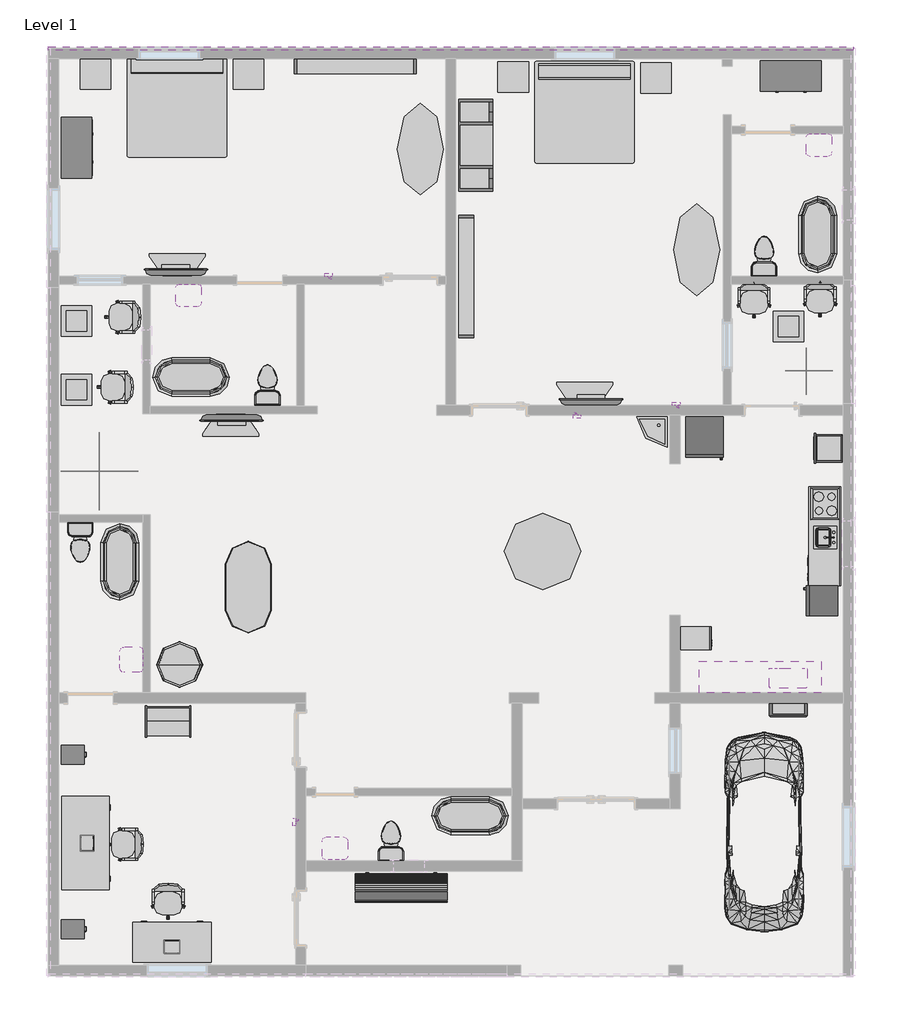
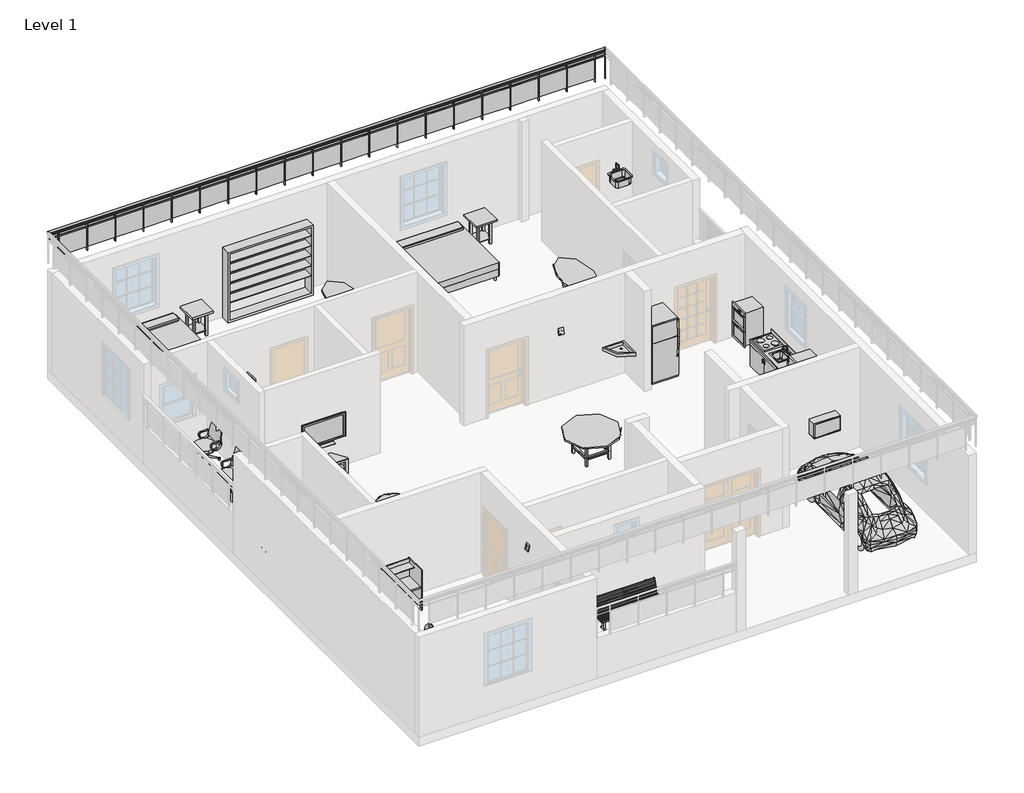
# One storey, part 4 of 4: 37 furniture elements, 17 proxies, 14 flow terminals, 3 geographic elements, 1 railing.
# Revit data of these elements (continued)
# Type "Shelving : 96\" x 12\" x 84\"" (continued)
#   Shelving Unit Material = Laminate, Ivory, Matte
#   Default Elevation = 0
# Type "TV - Flat Screen : 50\""
#   SinAng = 0' - 0.0193"
#   L = 3' - 7.57782"
#   H = 2' - 0.51477"
#   Thickness = 0' - 4.33071"
#   Diagonal = 4' - 2"
#   CosAng = 0' - 0.03431"
#   Stand [instance default] = yes
#   Default Elevation = 0
# Type "TV Stand : TV Stand"
#   Depth = 1' - 6"
#   Width = 3' - 8"
#   Height = 1' - 7 1/2"
#   Finish = Melamine - Gray
#   Default Elevation = 0
# Type "Table-Coffee : 24\" x 24\" x 24\""
#   Assembly Code = "E2020200"
#   Height = 2' - 0"
#   Length = 2' - 0"
#   Width = 2' - 0"
#   Top Material = none
#   Frame Material = none
#   Default Elevation = 0
# Type "Table-Dining Oval : 36\" x 72\""
#   Assembly Code = "E2020200"
#   Length = 6' - 0"
#   Width = 3' - 0"
#   Base Material = Steel, Chrome Plated
#   Top Material = Glass - Clear, Grey
#   Default Elevation = 0
#   Description = (empty or 0)
# Type "Table-Dining Round w Chairs : 60\" Diameter"
#   Assembly Code = "E2020200"
#   Radius = 2' - 6"
#   Diameter = 5' - 0"
#   Height = 2' - 6"
#   Chairs = 6
#   Base Material = Pine
#   Top Material = Laminate, Linen, Matte
#   Default Elevation = 0
# Type "Table-Ellipse : 72\" x 36\""
#   Assembly Code = "E2020200"
#   Half Width = 1' - 6"
#   Half Length = 3' - 0"
#   Height = 2' - 6"
#   Length = 6' - 0"
#   Width = 3' - 0"
#   Base Material = Birch
#   Top Material = Laminate - Black
#   Default Elevation = 0
# Type "Table-Night Stand : 24\" x 24\" x 30\""
#   Assembly Code = "E2020200"
#   Depth = 2' - 0"
#   Height = 2' - 6"
#   Width = 2' - 0"
#   Base Material = Birch
#   Top Material = Laminate, Ivory, Matte
#   Default Elevation = 0
# Type "Table-Round : 36\" Diameter"
#   Assembly Code = "E2020200"
#   Base Radius = 0' - 10"
#   Height = 2' - 6"
#   Radius = 1' - 6"
#   Base Material = Steel, Chrome Plated
#   Top Material = Birch
#   Default Elevation = 0
# Type "Park Bench : 72\""
#   Length = 6' - 0"
#   Seat Material = Wood - Teak
#   Frame Material = Steel, Paint Finish, Dark Gray, Matte
# Type "RPC Shrub : Burning Bush 4'-6\""
#   Type Comments = "Burning Bush"
#   built-in parameter 1005198 = "{2, 15},{39, RPC-16-FVGW-0UXX-7JA7-N000-ST1L-LVER-AU},{1, 0},{1, 0},{2, 13},{1, 8},{5, Color},{1, 0},{1, 0},{3, 0.8},{3, 0.8},{3, 0.8},{1, 8},{7, BBoxMin},{1, 0},{1, 0},{1, 0},{1, 0},{1, 0},{1, 8},{7, BBoxMax},{1, 0},{1, 0},{1, 0},{1, 0},{1, 0},{2, 11},{9, RPCTypeId},{1, 0},{1, 0},{39, RPC-16-FVGW-0UXX-7JA7-N000-ST1L-LVER-AU},{1, 6},{14, RPCPlantHeight},{1, 0},{1, 0},{3, 4.5},{2, 11},{7, keyword},{1, 0},{1, 0},{35, :RPCs:Shrubs & Grasses:Geometry:RPC},{2, 11},{8, category},{1, 0},{1, 0},{16, Shrubs & Grasses},{2, 11},{12, LocalizedUID},{1, 0},{1, 0},{12, Burning Bush},{2, 14},{6, Height},{1, 0},{1, 0},{3, 4.5},{1, 2},{16, Cast Reflections},{1, 0},{1, 0},{1, 0},{1, 2},{12, Cast Shadows},{1, 0},{1, 0},{1, 1},{1, 2},{9, Lock View},{1, 0},{1, 0},{1, 0},{1, 4},{5, ViewC},{1, 0},{1, 0},{1, 0},{21, assetlibrary_base.fbx},{1, 5},"
#   built-in parameter 1005195 = "RPC-16-FVGW-0UXX-7JA7-N000-ST1L-LVER-AU"
#   Assembly Code = "G2050500"
#   Height = 4' - 6"
#   Default Elevation = 0
# Type "RPC Shrub : Cedar Shrub 3'-0\""
#   Type Comments = "Cedar Shrub"
#   built-in parameter 1005198 = "{2, 15},{39, RPC-16-FUMD-ULXX-U7X6-J000-ST1L-LVER-AU},{1, 0},{1, 0},{2, 13},{1, 8},{5, Color},{1, 0},{1, 0},{3, 0.8},{3, 0.8},{3, 0.8},{1, 8},{7, BBoxMin},{1, 0},{1, 0},{1, 0},{1, 0},{1, 0},{1, 8},{7, BBoxMax},{1, 0},{1, 0},{1, 0},{1, 0},{1, 0},{2, 11},{9, RPCTypeId},{1, 0},{1, 0},{39, RPC-16-FUMD-ULXX-U7X6-J000-ST1L-LVER-AU},{1, 6},{14, RPCPlantHeight},{1, 0},{1, 0},{1, 3},{2, 11},{7, keyword},{1, 0},{1, 0},{35, :RPCs:Shrubs [General]:Geometry:RPC},{2, 11},{8, category},{1, 0},{1, 0},{16, Shrubs [General]},{2, 11},{12, LocalizedUID},{1, 0},{1, 0},{11, Cedar Shrub},{2, 14},{6, Height},{1, 0},{1, 0},{1, 3},{1, 2},{16, Cast Reflections},{1, 0},{1, 0},{1, 0},{1, 2},{12, Cast Shadows},{1, 0},{1, 0},{1, 1},{1, 2},{9, Lock View},{1, 0},{1, 0},{1, 0},{1, 4},{5, ViewC},{1, 0},{1, 0},{1, 0},{21, assetlibrary_base.fbx},{1, 5},"
#   built-in parameter 1005195 = "RPC-16-FUMD-ULXX-U7X6-J000-ST1L-LVER-AU"
#   Assembly Code = "G2050500"
#   Height = 3' - 0"
#   Default Elevation = 0
# Type "Glass Panel - Bottom Fill"
#   Assembly Code = "C2010400"
#   built-in parameter 1008612 = 0.0416667 (stored number, unit not read)
#   built-in parameter 1008611 = 0.0416667 (stored number, unit not read)
#   built-in parameter 1008609 = 0.333333 (stored number, unit not read)
#   built-in parameter 1008604 = 0.166667 (stored number, unit not read)
#   built-in parameter 1008603 = 0.166667 (stored number, unit not read)
#   Railing Height = 3' - 0"
#   built-in parameter 1008630 = 2
#   built-in parameter 1008610 = 2
#   built-in parameter 1008618 = Baluster - Square : 3/4"
# Elements 1, 2 (IfcBuildingElementProxy)
#   Phase Created = New Construction
# Element 3 (IfcBuildingElementProxy, "18\" x 24\" x 34 1/2\"")
#   Phase Created = New Construction
#   Materials on its faces: "Steel, Paint Finish, Ivory, Matte", "Plastic, Opaque Black"
# Element 4 (IfcBuildingElementProxy, "Cook Top-4 Unit2 : 22\" x 20\"")
#   Phase Created = New Construction
#   Materials on its faces: "Steel, Chrome Plated", "Steel, Polished"
# Element 5 (IfcBuildingElementProxy, "Dishwasher : 24\" x 24\" x 34\"")
#   Phase Created = New Construction
#   Materials on its faces: "Steel, Paint Finish, Ivory, Glossy", "Plastic, Opaque Black"
# Element 6 (IfcBuildingElementProxy, "Kitchenette - Medium : Kitchenette - Medium")
#   Phase Created = New Construction
#   Materials on its faces: "Cabinets", "Cabinets - Handles"
# Elements 7, 8 (IfcBuildingElementProxy, "Microwave : 30\" x 16\" x 18\"")
#   Phase Created = New Construction
#   Materials on its faces: "Laminate, Ivory, Matte", "Glass"
# Element 9 (IfcBuildingElementProxy, "Oven Double-Built-in : 21 1/2\" x 39 1/4\" x 21\"")
#   Phase Created = New Construction
#   Materials on its faces: "Steel", "Metal - Stainless Steel, Polished", "Glass"
# Element 10 (IfcBuildingElementProxy, "RPC Beetle : RPC Beetle")
#   Phase Created = New Construction
# Elements 11, 12, 13, 14 (IfcBuildingElementProxy, "RPC Picture Frame : RPC Picture Frame")
#   Phase Created = New Construction
# Element 15 (IfcBuildingElementProxy, "Refrigerator : 24\" x 25\" LH")
#   Phase Created = New Construction
#   Materials on its faces: "Steel, Paint Finish, Ivory, Glossy", "Steel, Chrome Plated"
# Element 16 (IfcBuildingElementProxy, "Refrigerator.0001 : 30\" x 32\" RH")
#   Phase Created = New Construction
#   Materials on its faces: "Steel, Paint Finish, Ivory, Glossy", "Steel, Chrome Plated"
# Element 17 (IfcBuildingElementProxy, "Single Carrel : Single Carrel")
#   Phase Created = New Construction
#   Materials on its faces: "Laminate, Ivory, Matte", "Cherry"
# Element 18 (IfcFlowTerminal, "Sink - Corner Floor : 24\"")
#   Mark = "14"
#   Phase Created = New Construction
# Element 19 (IfcFlowTerminal, "Sink Kitchen-Island : 18\" x 18\"")
#   Mark = "15"
#   Phase Created = New Construction
#   Materials on its faces: "Steel, Polished"
# Element 20 (IfcFlowTerminal, "Sink Vanity-Square : 20\" x 18\"")
#   Mark = "1"
#   Phase Created = New Construction
#   Materials on its faces: "Porcelain, Linen", "Steel, Polished"
# Element 21 (IfcFlowTerminal, "Sink Vanity-Square : 20\" x 18\"")
#   Mark = "2"
#   Phase Created = New Construction
#   Materials on its faces: "Porcelain, Linen", "Steel, Polished"
# Element 22 (IfcFlowTerminal, "Sink Vanity-Square : 20\" x 18\"")
#   Mark = "9"
#   Phase Created = New Construction
#   Materials on its faces: "Porcelain, Linen", "Steel, Polished"
# Element 23 (IfcFlowTerminal, "Sink Vanity-Square : 20\" x 18\"")
#   Mark = "16"
#   Phase Created = New Construction
#   Materials on its faces: "Porcelain, Linen", "Steel, Polished"
# Element 24 (IfcFlowTerminal, "Toilet-Domestic-3D : Toilet-Domestic-3D")
#   Mark = "6"
#   Phase Created = New Construction
#   Materials on its faces: "Porcelain, Linen", "Laminate, Linen, Matte"
# Element 25 (IfcFlowTerminal, "Toilet-Domestic-3D : Toilet-Domestic-3D")
#   Mark = "7"
#   Phase Created = New Construction
#   Materials on its faces: "Porcelain, Linen", "Laminate, Linen, Matte"
# Element 26 (IfcFlowTerminal, "Toilet-Domestic-3D : Toilet-Domestic-3D")
#   Mark = "8"
#   Phase Created = New Construction
#   Materials on its faces: "Porcelain, Linen", "Laminate, Linen, Matte"
# Element 27 (IfcFlowTerminal, "Toilet-Domestic-3D : Toilet-Domestic-3D")
#   Mark = "19"
#   Phase Created = New Construction
#   Materials on its faces: "Porcelain, Linen", "Laminate, Linen, Matte"
# Element 28 (IfcFlowTerminal, "Tub-Free Standing-3D : 30\" x 60\"")
#   Mark = "3"
#   Phase Created = New Construction
#   Materials on its faces: "Porcelain, Ivory"
# Element 29 (IfcFlowTerminal, "Tub-Free Standing-3D : 30\" x 60\"")
#   Mark = "4"
#   Phase Created = New Construction
#   Materials on its faces: "Porcelain, Ivory"
# Element 30 (IfcFlowTerminal, "Tub-Free Standing-3D : 30\" x 60\"")
#   Mark = "11"
#   Phase Created = New Construction
#   Materials on its faces: "Porcelain, Ivory"
# Element 31 (IfcFlowTerminal, "Tub-Free Standing-3D : 30\" x 60\"")
#   Mark = "17"
#   Phase Created = New Construction
#   Materials on its faces: "Porcelain, Ivory"
# Elements 32, 33 (IfcFurniture, "Bed-Standard.0001 : King 78\" x 80\"")
#   Phase Created = New Construction
#   Materials on its faces: "Linen, White", "Steel, Chrome Plated"
# Elements 34, 35 (IfcFurniture, "Cabinet-File 5 Drawer : 15\" x 18\"")
#   Phase Created = New Construction
#   Materials on its faces: "Steel, Chrome Plated", "Steel, Paint Finish, Ivory, Glossy"
# Elements 36, 37, 38, 39, 40, 41 (IfcFurniture, "Chair-Executive : Chair-Executive")
#   Phase Created = New Construction
#   Materials on its faces: "Plastic, Opaque Black", "Textile - Slate Blue"
# Element 42 (IfcFurniture, "Counter Top w Sink Hole : 24\" Depth")
#   Sink Opening Width = 2' - 3"
#   Sink Opening Depth = 1' - 3"
#   Sink Location To Wall = 0' - 6"
#   Sink Location = 2' - 0"
#   Length = 8' - 0"
#   Phase Created = New Construction
#   Materials on its faces: "Counter Top"
# Element 43 (IfcFurniture, "Counter Top w Sink Hole : 24\" Depth")
#   Sink Opening Depth = 1' - 2"
#   Sink Location To Wall = 0' - 6"
#   Length = 6' - 6"
#   Sink Location = 3' - 4"
#   Sink Opening Width = 1' - 4"
#   Phase Created = New Construction
#   Materials on its faces: "Counter Top"
# Element 44 (IfcFurniture, "Desk : 60\" x 30\" Student")
#   Phase Created = New Construction
#   Materials on its faces: "Steel, Chrome Plated", "Laminate, Ivory, Matte", "Cherry"
# Element 45 (IfcFurniture, "Desk : 72\" x 36\"")
#   Phase Created = New Construction
#   Materials on its faces: "Steel, Chrome Plated", "Laminate, Ivory, Matte", "Cherry"
# Elements 46, 47 (IfcFurniture, "Dresser : 48\" x 72\" x 24\"")
#   Phase Created = New Construction
#   Materials on its faces: "Laminate, Ivory, Matte", "Cherry", "Laminate - Ivory, Glossy"
# Element 48 (IfcFurniture, "Entertainment Center : 72\" x 72\" x 24\"")
#   Phase Created = New Construction
#   Materials on its faces: "Steel, Chrome Plated", "Glass - Clear, Grey"
# Elements 49, 50 (IfcFurniture, "Shelving : 96\" x 12\" x 84\"")
#   Phase Created = New Construction
#   Materials on its faces: "Laminate, Ivory, Matte"
# Elements 51, 52, 53 (IfcFurniture, "TV - Flat Screen : 50\"")
#   Stand = yes
#   Phase Created = New Construction
#   Materials on its faces: "TV - Black", "TV - Glass", "TV - Screen"
# Elements 54, 55, 56 (IfcFurniture, "TV Stand : TV Stand")
#   Phase Created = New Construction
#   Materials on its faces: "Melamine - Gray", "Glass - Shelves"
# Elements 57, 58, 59 (IfcFurniture, "Table-Coffee : 24\" x 24\" x 24\"")
#   Phase Created = New Construction
#   Materials on its faces: "Glass - Clear, Grey"
# Element 60 (IfcFurniture, "Table-Dining Oval : 36\" x 72\"")
#   Phase Created = New Construction
#   Materials on its faces: "Steel, Chrome Plated", "Glass - Clear, Grey"
# Element 61 (IfcFurniture, "Table-Dining Round w Chairs : 60\" Diameter")
#   Phase Created = New Construction
#   Materials on its faces: "Pine", "Laminate, Linen, Matte"
# Elements 62, 63 (IfcFurniture, "Table-Ellipse : 72\" x 36\"")
#   Phase Created = New Construction
#   Materials on its faces: "Birch", "Laminate - Black"
# Elements 64, 65, 66, 67 (IfcFurniture, "Table-Night Stand : 24\" x 24\" x 30\"")
#   Phase Created = New Construction
#   Materials on its faces: "Birch", "Laminate, Ivory, Matte"
# Element 68 (IfcFurniture, "Table-Round : 36\" Diameter")
#   Phase Created = New Construction
#   Materials on its faces: "Steel, Chrome Plated", "Birch"
# Element 69 (IfcGeographicElement, "Park Bench : 72\"")
#   Phase Created = New Construction
#   Materials on its faces: "Wood - Teak", "Steel, Paint Finish, Dark Gray, Matte"
# Element 70 (IfcGeographicElement, "RPC Shrub : Burning Bush 4'-6\"")
#   Phase Created = New Construction
# Element 71 (IfcGeographicElement, "RPC Shrub : Cedar Shrub 3'-0\"")
#   Phase Created = New Construction
# Element 72 (IfcRailing, "Glass Panel - Bottom Fill")
#   built-in parameter 1008621 = 10.6667 (stored number, unit not read)
#   Phase Created = New Construction
#   Materials on its faces: "Glass"
# Materials
#   "Plastic, Opaque Black": class "Plastic", colour RGB 0 0 0, transparency 0, Description = "Plastic, generic, opaque black", Cost = 0
#   "Steel, Paint Finish, Ivory, Matte": class "Metal", colour RGB 247 247 239, transparency 0, Description = "Steel, paint finish, ivory, matte", Cost = 0
#   "Steel, Chrome Plated": class "Metal", colour RGB 17 17 17, transparency 0, Description = "Chromiuim plated steel", Cost = 0
#   "Steel, Polished": class "Metal", colour RGB 57 57 57, transparency 0, Description = "Polished steel", Cost = 0
#   "Steel, Paint Finish, Ivory, Glossy": class "Metal", colour RGB 247 247 239, transparency 0, Description = "Steel, paint finish, ivory, glossy", Cost = 0
#   "Cabinets": colour RGB 249 249 249, transparency 0
#   "Cabinets - Handles": class "Metal", colour RGB 57 57 57, transparency 0
#   "Laminate, Ivory, Matte": class "Plastic", colour RGB 247 247 239, transparency 0, Description = "Plastic Laminate - Ivory, Matte", Cost = 0
#   "Metal - Stainless Steel, Polished": class "Metal", colour RGB 216 216 216, transparency 0
#   "Cherry": class "Wood", colour RGB 226 177 128, transparency 0, Description = "Prunus Serotina", Cost = 0
#   "Porcelain, Linen": class "Ceramic", colour RGB 249 239 230, transparency 0, Description = "Porcelain, linen", Cost = 0
#   "Laminate, Linen, Matte": class "Plastic", colour RGB 249 239 230, transparency 0, Description = "Plastic Laminate - Linen, Matte", Cost = 0
#   "Porcelain, Ivory": class "Ceramic", colour RGB 247 247 239, transparency 0, Description = "Porcelain, ivory", Cost = 0
#   "Linen, White": class "Textile", colour RGB 247 247 239, transparency 0, Description = "Linen, white", Cost = 0
#   "Textile - Slate Blue": class "Fabric", colour RGB 98 102 118, transparency 0
#   "Laminate - Ivory, Glossy": colour RGB 247 247 239, transparency 0
#   "Melamine - Gray": class "Wood", colour RGB 49 49 49, transparency 0
#   "Glass - Clear, Grey": class "Glass", colour RGB 252 255 255, transparency 0.64
#   "Pine": class "Wood", colour RGB 223 192 134, transparency 0, Description = "Pinus Echinata", Cost = 0
#   "Birch": class "Wood", colour RGB 224 178 126, transparency 0, Description = "Betula Alleghaniensis", Cost = 0
#   "Laminate - Black": colour RGB 0 0 0, transparency 0
#   "Wood - Teak": class "Wood", colour RGB 145 112 90, transparency 0
#   "Steel, Paint Finish, Dark Gray, Matte": class "Metal", colour RGB 98 98 98, transparency 0, Description = "Steel, paint finish, dark gray, matte", Cost = 0
#   "Glass": class "Glass", colour RGB 0 128 192, transparency 0.75, Description = "Soda Lime Glass", Cost = 0
#   "Steel": class "Metal", colour RGB 247 247 247, transparency 0, Description = "Steel, mill finish", Cost = 0
#   "Counter Top": class "Wood", colour RGB 226 177 128, transparency 0
#   "TV - Black": colour RGB 49 49 49, transparency 0
#   "TV - Glass": colour RGB 157 157 157, transparency 0.9
#   "TV - Screen": colour RGB 0 0 0, transparency 0
#   "Glass - Shelves": class "Glass", colour RGB 167 167 167, transparency 0.9
